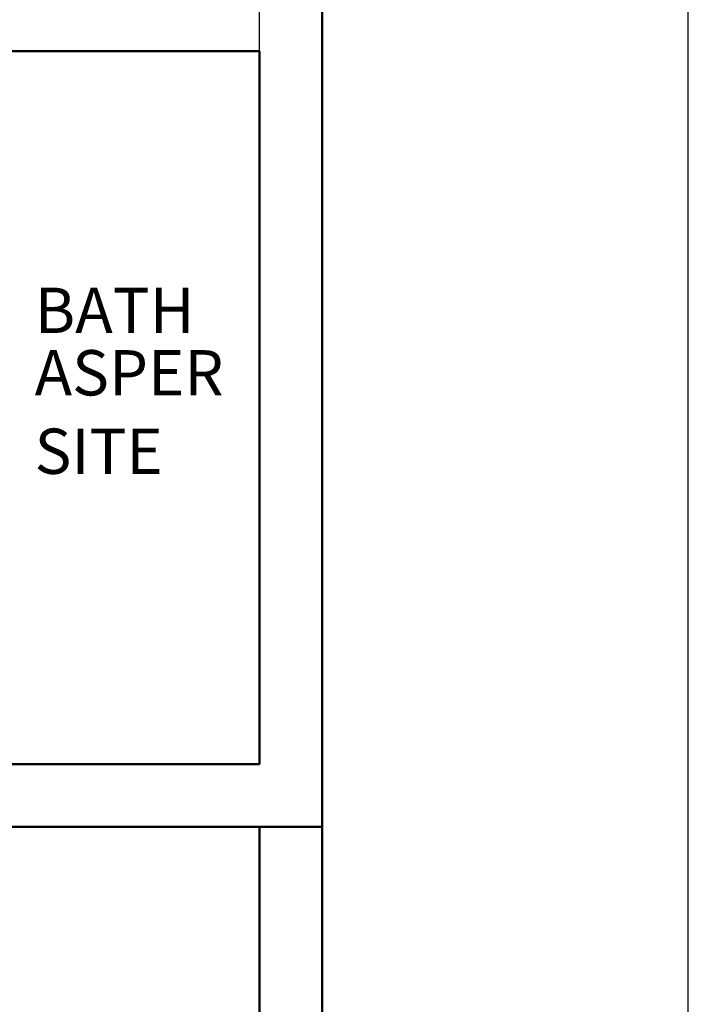
# Model space of a CAD drawing. Units: inches. Extents: x 5375 to 6084, y 16106 to 17259.
# Tile 14 of 32: x 5988 to 6084, y 16377 to 16518. Entities that reach past the tile are written whole.
import ezdxf

# ---------------------------------------------------------------- set-up
doc = ezdxf.new("R2010")
doc.units = ezdxf.units.IN
for name, color, linetype, lineweight in [('A-ANNO-DIMS', 2, 'Continuous', 18), ('A-AREA-IDEN', 5, 'Continuous', 18), ('WALL', 6, 'Continuous', 50)]:
    doc.layers.add(name, color=color, linetype=linetype, lineweight=lineweight)
doc.styles.get("Standard").update_dxf_attribs({"font": 'arial.ttf'})
doc.dimstyles.get("Standard").update_dxf_attribs({"dimtxt": 0.18, "dimasz": 0.18, "dimexe": 0.18, "dimexo": 0.0625, "dimgap": 0.09, "dimtad": 0, "dimtih": 1, "dimtoh": 1, "dimdec": 4, "dimzin": 0, "dimdsep": 46, "dimtxsty": 'Standard', "dimcen": 0.09, "dimadec": 0, "dimazin": 0, "dimtfac": 1, "dimtdec": 4, "dimtofl": 0, "dimtmove": 0, "dimatfit": 3, "dimfxl": 1, "dimtolj": 1, "dimtzin": 0, "dimarcsym": 0})

# ---------------------------------------------------------------- blocks, each defined once
blk = doc.blocks.new('*D31')
at = {"layer": 'A-ANNO-DIMS', "color": 0, "lineweight": -2, "transparency": 16777216}
for p, q in [((6031.68, 17206.58), (6084.2, 17206.58)), ((6084.02, 17206.4), (6084.02, 16709.66)), ((6084.02, 16212.56), (6084.02, 16709.3)), ((6031.68, 16212.38), (6084.2, 16212.38))]:
    blk.add_line(p, q, dxfattribs=at)
at = {"layer": 'A-ANNO-DIMS', "color": 0, "transparency": 16777216}
for points in [[(6083.99, 17206.4), (6084.05, 17206.4), (6084.02, 17206.58)], [(6083.99, 16212.56), (6084.05, 16212.56), (6084.02, 16212.38)]]:
    blk.add_solid(points, dxfattribs=at)
at = {"layer": 'Defpoints', "color": 0, "transparency": 16777216}
for p in [(6031.62, 17206.58), (6084.02, 17206.58), (6031.62, 16212.38)]:
    blk.add_point(p, dxfattribs=at)
at = {"layer": 'A-ANNO-DIMS', "color": 0, "transparency": 16777216, "insert": (6084.02, 16709.48), "char_height": 0.18, "attachment_point": 5}
blk.add_mtext('\\A1;994.2', dxfattribs=at)
blk = doc.blocks.new('*D48')
at = {"layer": 'A-ANNO-DIMS', "color": 0, "lineweight": -2, "transparency": 16777216}
for p, q in [((5962.62, 16411.64), (5962.62, 17259.16)), ((5962.8, 17258.98), (5992.4, 17258.98)), ((6022.44, 17258.98), (5992.84, 17258.98)), ((6022.62, 16411.64), (6022.62, 17259.16))]:
    blk.add_line(p, q, dxfattribs=at)
at = {"layer": 'A-ANNO-DIMS', "color": 0, "transparency": 16777216}
for points in [[(5962.8, 17259.01), (5962.8, 17258.95), (5962.62, 17258.98)], [(6022.44, 17259.01), (6022.44, 17258.95), (6022.62, 17258.98)]]:
    blk.add_solid(points, dxfattribs=at)
at = {"layer": 'Defpoints', "color": 0, "transparency": 16777216}
for p in [(6022.62, 17258.98), (5962.62, 16411.58), (6022.62, 16411.58)]:
    blk.add_point(p, dxfattribs=at)
at = {"layer": 'A-ANNO-DIMS', "color": 0, "transparency": 16777216, "insert": (5992.62, 17258.98), "char_height": 0.18, "attachment_point": 5}
blk.add_mtext('\\A1;60', dxfattribs=at)

msp = doc.modelspace()

# ---------------------------------------------------------------- linework, layer by layer
at = {"layer": 'WALL'}
for p, q in [((6031.6199, 16699.5793), (6031.6199, 16212.3785)), ((6031.6199, 16699.5793), (6031.6199, 16513.5793)), ((5791.6199, 16513.5793), (6022.6199, 16513.5793)), ((6022.6199, 16513.5793), (6022.6199, 16411.5793)), ((5761.6199, 16411.5793), (6022.6199, 16411.5793)), ((5761.6199, 16402.5793), (6031.6199, 16402.5793)), ((6022.6199, 16402.5793), (6022.6199, 16221.3785))]:
    msp.add_line(p, q, dxfattribs=at)

# ---------------------------------------------------------------- texts
at = {"layer": 'A-AREA-IDEN'}
for s, p in [('BATH', (5990.432, 16473.2551)), ('ASPER', (5990.432, 16464.322)), ('SITE', (5990.432, 16453.0983))]:
    msp.add_text(s, height=6.47981, dxfattribs=at).set_placement(p)

# ---------------------------------------------------------------- dimensions: what is measured, and where the dimension line sits
at = {"layer": 'A-ANNO-DIMS'}
dim = msp.add_linear_dim(base=(6022.6199, 17258.9793), p1=(5962.6199, 16411.5793), p2=(6022.6199, 16411.5793), dimstyle='Standard', override={"dimdec": 0, "dimlfac": 1, "dimrnd": 0, "dimzin": 0, "dimdsep": 46, "dimlunit": 2}, dxfattribs=at)
dim.commit()
dim.dimension.update_dxf_attribs({"geometry": '*D48', "text_midpoint": (5992.6199, 17258.9793)})
dim = msp.add_linear_dim(base=(6084.0199, 17206.5793), p1=(6031.6199, 16212.3785), p2=(6031.6199, 17206.5793), angle=90, dimstyle='Standard', override={"dimdec": 1, "dimlfac": 1, "dimrnd": 0, "dimzin": 0, "dimdsep": 46, "dimlunit": 2}, dxfattribs=at)
dim.commit()
dim.dimension.update_dxf_attribs({"geometry": '*D31', "text_midpoint": (6084.0199, 16709.4789)})

doc.saveas('drawing.dxf')
